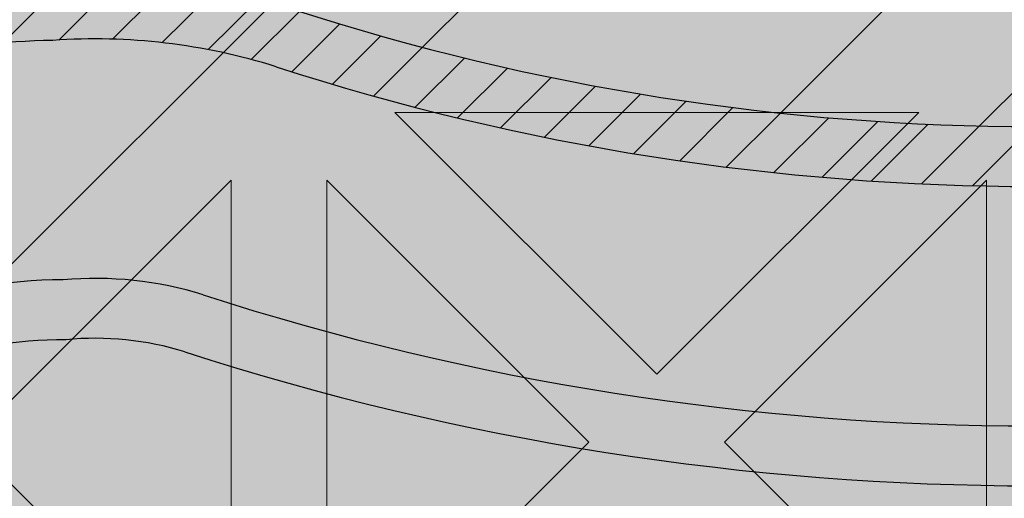
# Model space of a CAD drawing. Units: inches. Extents: x 844 to 2234, y 346 to 1084.
# Tile 54 of 93: x 1866.641 to 1869.26, y 692.527 to 693.802. Entities that reach past the tile are written whole.
import ezdxf

# ---------------------------------------------------------------- set-up
doc = ezdxf.new("R2010")
doc.units = ezdxf.units.IN
doc.header["$MEASUREMENT"] = 0
doc.layers.add('furniture', color=8, linetype='Continuous', lineweight=18)
doc.layers.add('RA-AP-01$0$INT', color=35, linetype='Continuous', lineweight=5)
doc.layers.add('RA-AP-01$0$FURN', color=3, linetype='Continuous')
doc.layers.add('RA-AP-01$0$WOOD', color=64, linetype='Continuous')

# ---------------------------------------------------------------- blocks, each defined once
blk = doc.blocks.new('A$C18D01794')
at = {"layer": 'RA-AP-01$0$INT'}
h = blk.add_hatch(color=256, dxfattribs=at)
h.paths.add_polyline_path([(4.585917135068449, -6.356712009588271), (4.555206456959269, -6.35671200958746), (4.555206456959137, -6.387422687716308), (4.874495778835233, -6.706712009592356), (4.90520645695423, -6.676001331474049)])
h.paths.add_polyline_path([(5.255206456948813, -6.387422687716306), (5.255206456948682, -6.356712009605972), (5.224495778822613, -6.356712009605161), (4.905206456953498, -6.676001331474273), (4.935917135072151, -6.706712009592924)])
h.paths.add_polyline_path([(4.935917135072559, -6.706712009592068), (4.905206456953564, -6.737422687710376), (5.255206456951813, -7.087422687708613), (5.255206456951549, -7.026001331471008)])
h.paths.add_polyline_path([(4.555206456956399, -7.026001331471013), (4.555206456956134, -7.087422687708616), (4.905206456953821, -6.737422687710943), (4.874495778835166, -6.70671200959229)])
h = blk.add_hatch(color=256, dxfattribs=at)
h.paths.add_polyline_path([(4.585917135068448, -6.356712009588273), (4.614201406330596, -6.356712009589021), (4.668846067270487, -6.411356670531338), (4.723490728212344, -6.356712009591912), (4.771774999457151, -6.35671200959319), (4.826419660396886, -6.411356670535356), (4.862780050090322, -6.374996280843536), (4.844495778842715, -6.356712009595112), (4.862780050090411, -6.356712009595595), (4.905206456960182, -6.399138416468211), (4.947632863832445, -6.356712009597838), (4.965917135079675, -6.356712009598322), (4.947632863831759, -6.374996280845421), (4.983993253523576, -6.411356670538857), (5.038637914464627, -6.356712009600247), (5.08692218571208, -6.356712009601523), (5.141566846649976, -6.411356670541852), (5.196211507589851, -6.356712009604411), (5.224495778822615, -6.356712009605161), (4.905206456953975, -6.676001331473793)])
h.paths.add_polyline_path([(4.895206456956031, -6.637717060225675), (4.895206456958921, -6.528427738347902), (4.840561796018589, -6.583072399285802)], flags=16)
h.paths.add_polyline_path([(4.915206456955638, -6.637717060226121), (4.969851117895509, -6.583072399288678), (4.915206456957609, -6.528427738348344)], flags=16)
h.paths.add_polyline_path([(4.826419660395175, -6.568930263661755), (4.881064321335613, -6.514285602723745), (4.771774999456703, -6.514285602720857)], flags=16)
h.paths.add_polyline_path([(4.983993253519558, -6.568930263665262), (5.038637914460456, -6.514285602726792), (4.929348592581548, -6.514285602724816)], flags=16)
h.paths.add_polyline_path([(4.881064321336025, -6.494285602723742), (4.826419660397532, -6.439640941782821), (4.771774999457062, -6.494285602720859)], flags=16)
h.paths.add_polyline_path([(4.929348592582019, -6.494285602724817), (5.038637914460982, -6.494285602726792), (4.983993253522945, -6.439640941786327)], flags=16)
h.paths.add_polyline_path([(4.895206456960191, -6.480143467100443), (4.895206456962115, -6.407422687715913), (4.876922185715016, -6.389138416467584), (4.840561796021581, -6.425498806159401)], flags=16)
h.paths.add_polyline_path([(4.915206456958487, -6.480143467100889), (4.969851117899527, -6.425498806162279), (4.933490728206909, -6.389138416468043), (4.9152064569598, -6.40742268771434)], flags=16)
h.paths.add_polyline_path([(4.757632863832376, -6.480143467096812), (4.812277524772842, -6.425498806158772), (4.757632863834348, -6.370854145217844)], flags=16)
h.paths.add_polyline_path([(4.737632863832376, -6.480143467096286), (4.737632863834348, -6.370854145217375), (4.682988202893906, -6.425498806155385)], flags=16)
h.paths.add_polyline_path([(5.05278005008503, -6.480143467103376), (5.052780050087917, -6.370854145224413), (4.998135389146995, -6.425498806162908)], flags=16)
h.paths.add_polyline_path([(5.072780050085024, -6.480143467103744), (5.127424711025931, -6.42549880616527), (5.072780050087916, -6.370854145224832)], flags=16)
h.paths.add_polyline_path([(4.935917135072783, -6.706712009592292), (5.255206456948811, -6.387422687716309), (5.255206456948932, -6.415706958964177), (5.200561796010279, -6.470351619902839), (5.255206456949403, -6.524996280841948), (5.25520645694961, -6.5732805520894), (5.200561796009787, -6.627925213029239), (5.236922185702417, -6.664285602721864), (5.255206456949919, -6.646001331474357), (5.255206456949998, -6.664285602721898), (5.212780050078687, -6.706712009592262), (5.25520645695036, -6.749138416463932), (5.255206456950438, -6.767422687711313), (5.236922185702424, -6.749138416463297), (5.200561796009796, -6.785498806155928), (5.255206456950753, -6.840143467096874), (5.25520645695096, -6.888427738341682), (5.200561796010322, -6.943072399282328), (5.255206456951428, -6.997717060223427), (5.255206456951547, -7.026001331471006)])
h.paths.add_polyline_path([(5.042988202883395, -6.785498806155427), (5.097632863823085, -6.840143467095101), (5.097632863822622, -6.730854145216193)], flags=16)
h.paths.add_polyline_path([(5.028846067259663, -6.771356670531693), (5.083490728198774, -6.716712009592573), (4.974201406321001, -6.716712009593042)], flags=16)
h.paths.add_polyline_path([(5.117632863823087, -6.840143467095186), (5.172277524762331, -6.785498806155926), (5.11763286382262, -6.730854145216225)], flags=16)
h.paths.add_polyline_path([(5.08349072819877, -6.696712009593886), (5.028846067259652, -6.642067348654775), (4.974201406320998, -6.696712009593438)], flags=16)
h.paths.add_polyline_path([(5.131774999446817, -6.854285602718917), (5.186419660386065, -6.799640941779662), (5.241064321325782, -6.854285602719365)], flags=17)
h.paths.add_polyline_path([(5.131774999446228, -6.716712009592374), (5.186419660386065, -6.771356670532194), (5.222780050079488, -6.734996280838764), (5.204495778832781, -6.716712009592063)], flags=16)
h.paths.add_polyline_path([(5.097632863822613, -6.682569873970264), (5.097632863823061, -6.573280552091354), (5.042988202883383, -6.627925213031044)], flags=16)
h.paths.add_polyline_path([(5.131774999446899, -6.874285602718915), (5.241064321325809, -6.874285602719364), (5.186419660386591, -6.928930263658598)], flags=17)
h.paths.add_polyline_path([(5.131774999446226, -6.696712009594078), (5.204495778830767, -6.696712009594374), (5.22278005007868, -6.67842773834687), (5.186419660386049, -6.642067348654249)], flags=16)
h.paths.add_polyline_path([(5.11763286382262, -6.682569873970225), (5.17227752476232, -6.627925213030515), (5.117632863823064, -6.573280552091267)], flags=16)
h.paths.add_polyline_path([(5.186419660386069, -6.613783077405491), (5.241064321325754, -6.559138416465795), (5.131774999446791, -6.559138416466263)], flags=16)
h.paths.add_polyline_path([(5.131774999446872, -6.539138416466263), (5.24106432132578, -6.539138416465794), (5.186419660386554, -6.484493755526573)], flags=16)
h.paths.add_polyline_path([(5.255206456951811, -7.08742268770861), (5.255206456951895, -7.106712009588038), (4.555206456956052, -7.106712009588038), (4.555206456956136, -7.087422687708617), (4.905206456953973, -6.737422687710788)])
h.paths.add_polyline_path([(4.983993253513404, -6.8444937555241), (4.92934859257295, -6.899138416462108), (5.03863791445186, -6.899138416465014)], flags=16)
h.paths.add_polyline_path([(4.969851117889988, -6.83035161990006), (4.915206456952556, -6.775706958960171), (4.915206456949648, -6.884996280837944)], flags=16)
h.paths.add_polyline_path([(4.929348592572535, -6.919138416462105), (4.983993253511019, -6.973783077403037), (5.038637914451496, -6.919138416465012)], flags=16)
h.paths.add_polyline_path([(5.052780050074912, -6.93328055208906), (4.998135389134438, -6.987925213027088), (5.052780050072919, -7.042569873968025)], flags=16)
h.paths.add_polyline_path([(5.07278005007491, -6.933280552089588), (5.072780050072918, -7.042569873968497), (5.127424711013374, -6.987925213030498)], flags=16)
h.paths.add_polyline_path([(4.89520645695295, -6.775706958959721), (4.840561796013067, -6.830351619897157), (4.895206456950961, -6.884996280837494)], flags=16)
h.paths.add_polyline_path([(4.915206456948365, -6.933280552085403), (4.915206456946434, -7.006001331471951), (4.933490728192729, -7.024285602719066), (4.969851117886972, -6.987925213026453)], flags=16)
h.paths.add_polyline_path([(4.881064321327021, -6.899138416461022), (4.82641966038902, -6.84449375552057), (4.771774999448108, -6.899138416459029)], flags=16)
h.paths.add_polyline_path([(4.895206456950073, -6.933280552084951), (4.840561796009022, -6.987925213023558), (4.876922185700835, -7.024285602716997), (4.895206456948749, -7.006001331469487)], flags=16)
h.paths.add_polyline_path([(4.983993253510392, -7.0020673486505), (4.947632863816944, -7.038427738342319), (4.965917135064043, -7.05671200959023), (5.038637914448995, -7.056712009591555)], flags=16)
h.paths.add_polyline_path([(4.881064321326543, -6.91913841646102), (4.771774999447578, -6.919138416459031), (4.826419660385607, -6.973783077399508)], flags=16)
h.paths.add_polyline_path([(4.905206456946447, -7.014285602717636), (4.862780050074785, -7.056712009588352), (4.947632863816685, -7.056712009589775)], flags=16)
h.paths.add_polyline_path([(5.14156684663679, -7.002067348654549), (5.086922185696452, -7.056712009592438), (5.196211507574223, -7.056712009594425)], flags=16)
h.paths.add_polyline_path([(4.8264196603837, -7.002067348646972), (4.771774999442643, -7.056712009585575), (4.8444957788276, -7.056712009587508), (4.862780050075511, -7.038427738340416)], flags=16)
h.paths.add_polyline_path([(4.812277524760289, -6.98792521302292), (4.757632863822258, -6.933280552082447), (4.757632863819352, -7.042569873961408)], flags=16)
h.paths.add_polyline_path([(4.73763286382226, -6.933280552082079), (4.682988202881349, -6.987925213020536), (4.737632863819352, -7.04256987396099)], flags=16)
h.paths.add_polyline_path([(4.723490728195188, -7.056712009584289), (4.668846067257299, -7.002067348643949), (4.614201406317417, -7.056712009581383)], flags=16)
h.paths.add_polyline_path([(4.597632863829262, -6.706712009592262), (4.555206456957951, -6.664285602721896), (4.555206456958029, -6.646001331474357), (4.573490728205535, -6.664285602721864), (4.609851117898167, -6.627925213029238), (4.555206456958338, -6.573280552089402), (4.555206456958546, -6.524996280841952), (4.60985111789767, -6.470351619902839), (4.555206456959015, -6.415706958964177), (4.555206456959138, -6.387422687716309), (4.874495778835167, -6.70671200959229), (4.5552064569564, -7.026001331471015), (4.555206456956523, -6.997717060223433), (4.609851117897629, -6.94307239928233), (4.555206456956988, -6.888427738341681), (4.555206456957198, -6.840143467096881), (4.609851117898153, -6.78549880615593), (4.573490728205528, -6.749138416463297), (4.555206456957507, -6.76742268771132), (4.555206456957585, -6.749138416463933)])
h.paths.add_polyline_path([(4.712780050085332, -6.730854145216195), (4.712780050084863, -6.840143467095105), (4.767424711024555, -6.785498806155427)], flags=16)
h.paths.add_polyline_path([(4.726922185709173, -6.716712009592573), (4.781566846648288, -6.771356670531693), (4.836211507586949, -6.716712009593043)], flags=16)
h.paths.add_polyline_path([(4.692780050085327, -6.730854145216225), (4.638135389145619, -6.785498806155928), (4.692780050084865, -6.840143467095185)], flags=16)
h.paths.add_polyline_path([(4.726922185709182, -6.696712009593886), (4.836211507586949, -6.696712009593436), (4.7815668466483, -6.642067348654773)], flags=16)
h.paths.add_polyline_path([(4.678637914461726, -6.71671200959237), (4.605917135075169, -6.716712009592063), (4.587632863828464, -6.734996280838766), (4.623993253521887, -6.771356670532195)], flags=16)
h.paths.add_polyline_path([(4.712780050085336, -6.68256987397026), (4.767424711024568, -6.627925213031042), (4.71278005008489, -6.573280552091352)], flags=16)
h.paths.add_polyline_path([(4.678637914461726, -6.696712009594076), (4.623993253521899, -6.642067348654247), (4.587632863829271, -6.67842773834687), (4.605917135077185, -6.696712009594376)], flags=16)
h.paths.add_polyline_path([(4.692780050085336, -6.682569873970228), (4.692780050084889, -6.573280552091267), (4.638135389145632, -6.627925213030515)], flags=16)
h.paths.add_polyline_path([(4.623993253521885, -6.799640941779662), (4.678637914461131, -6.854285602718915), (4.56934859258217, -6.854285602719365)], flags=17)
h.paths.add_polyline_path([(4.623993253521901, -6.613783077405509), (4.678637914461158, -6.559138416466263), (4.569348592582195, -6.559138416465795)], flags=16)
h.paths.add_polyline_path([(4.678637914461051, -6.874285602718915), (4.623993253521361, -6.928930263658598), (4.569348592582143, -6.874285602719364)], flags=17)
h.paths.add_polyline_path([(4.678637914461076, -6.539138416466263), (4.623993253521399, -6.484493755526573), (4.569348592582167, -6.539138416465796)], flags=16)
h = blk.add_hatch(color=256, dxfattribs=at)
h.paths.add_polyline_path([(4.969851117891331, -6.583072399286455), (4.915206456952669, -6.63771706022511), (4.915206456952222, -6.528427738347337)])
h.paths.add_polyline_path([(4.895206456953064, -6.637717060225108), (4.840561796014413, -6.583072399286448), (4.895206456953533, -6.528427738347335)])
h.paths.add_polyline_path([(4.826419660390684, -6.568930263662714), (4.771774999451003, -6.514285602723024), (4.881064321329913, -6.514285602723489)])
h.paths.add_polyline_path([(4.881064321329884, -6.494285602723492), (4.771774999450921, -6.494285602723024), (4.82641966039018, -6.439640941783778)])
h.paths.add_polyline_path([(4.895206456953734, -6.48014346709988), (4.840561796013912, -6.425498806160046), (4.876922185707337, -6.389138416466622), (4.895206456954043, -6.40742268771333)])
h.paths.add_polyline_path([(4.862780050082808, -6.374996280843689), (4.826419660390178, -6.411356670536314), (4.771774999450351, -6.356712009596481), (4.844495778835303, -6.356712009596181)])
h.paths.add_polyline_path([(4.812277524766446, -6.425498806160041), (4.757632863827191, -6.480143467099289), (4.757632863826741, -6.370854145220329)])
h.paths.add_polyline_path([(4.737632863827191, -6.480143467099214), (4.682988202887508, -6.425498806159518), (4.737632863826743, -6.370854145220299)])
h.paths.add_polyline_path([(4.668846067263777, -6.41135667053579), (4.614201406325123, -6.356712009597128), (4.723490728202894, -6.356712009596675)])
h.paths.add_polyline_path([(4.905206456953846, -6.399138416467422), (4.862780050082654, -6.356712009596229), (4.947632863824561, -6.356712009595756)])
h.paths.add_polyline_path([(4.915206456952028, -6.480143467099882), (4.91520645695173, -6.407422687715346), (4.933490728199234, -6.389138416467428), (4.96985111789186, -6.425498806160055)])
h.paths.add_polyline_path([(5.038637914454841, -6.494285602723048), (4.929348592575874, -6.494285602723497), (4.983993253515593, -6.439640941783787)])
h.paths.add_polyline_path([(4.983993253515065, -6.568930263662725), (4.929348592575849, -6.514285602723495), (5.038637914454755, -6.514285602723045)])
h.paths.add_polyline_path([(5.052780050079843, -6.480143467099317), (4.998135389140595, -6.425498806160058), (5.052780050080309, -6.370854145220356)])
h.paths.add_polyline_path([(4.983993253516868, -6.411356670536324), (4.947632863824241, -6.374996280843694), (4.965917135071747, -6.356712009596188), (5.038637914456701, -6.356712009596504)])
h.paths.add_polyline_path([(5.127424711019533, -6.425498806159557), (5.072780050079843, -6.480143467099239), (5.07278005008031, -6.370854145220326)])
h.paths.add_polyline_path([(5.141566846643269, -6.411356670535829), (5.086922185704154, -6.356712009596707), (5.196211507581929, -6.356712009597176)])
for p, q in [((4.905206456953975, -6.676001331473793), (4.585917135071132, -6.356712009590955)), ((4.737632863834348, -6.370854145217375), (4.682988202893906, -6.425498806155385)), ((4.737632863832376, -6.480143467096285), (4.737632863834348, -6.370854145217375)), ((4.757632863832376, -6.48014346709681), (4.757632863834348, -6.370854145217847)), ((4.757632863834348, -6.370854145217847), (4.812277524772842, -6.425498806158774)), ((4.840561796021581, -6.425498806159403), (4.876922185715016, -6.389138416467584)), ((4.895206456962113, -6.407422687715495), (4.895206456960191, -6.480143467100447)), ((4.682988202893908, -6.425498806155387), (4.737632863832376, -6.480143467096285)), ((4.757632863832376, -6.48014346709681), (4.812277524772842, -6.425498806158774)), ((4.895206456960191, -6.480143467100447), (4.840561796021581, -6.425498806159401)), ((4.771774999457064, -6.494285602720857), (4.826419660397532, -6.439640941782821)), ((4.881064321336027, -6.494285602723744), (4.826419660397532, -6.439640941782821)), ((4.771774999457064, -6.494285602720857), (4.881064321336027, -6.494285602723744))]:
    blk.add_line(p, q, dxfattribs=at)
blk = doc.blocks.new('A$C32926AE1')
at = {"layer": 'RA-AP-01$0$WOOD'}
h = blk.add_hatch(color=256, dxfattribs=at)
h.dxf.hatch_style = 1
h.paths.add_polyline_path([(5.157430609644524, 4.573483066760929, -0.1009492694046607), (5.155401577623758, 4.593365984175333, -0.1842662638101597), (5.172249623284174, 4.638795604568598, 0.2056608120311276), (5.179560981299304, 4.661316324430096, 0.3614336704623542), (5.134352340494423, 4.706524965234944, 0.2056608120311297), (5.111831620632933, 4.699213607219793, -0.1842662638101113), (5.066402000239693, 4.682365561559342, -0.1055311479399994), (5.045656153913092, 4.68467289944697, 0.1567636581983829), (4.763886414745334, 4.684672899446966, -0.1055311479399895), (4.743140568418733, 4.68236556155934, -0.1842662638100833), (4.6977109480255, 4.69921360721979, 0.2056608120302612), (4.675190228164109, 4.706524965234949, 0.3614336704708441), (4.629981587358889, 4.66131632442871, 0.2056608120245944), (4.637292945374126, 4.638795604567974, -0.1842662638101024), (4.654140991034615, 4.59336598417475, -0.1009492694055169), (4.652111959013835, 4.573483066760181, 0.021410119221476), (4.629748025606143, 4.156712009541676, 0.0214101192214795), (4.652111959013809, 3.739940952323101, -0.1009492694059586), (4.654140991034615, 3.720058034908448, -0.1842662638100975), (4.637292945374126, 3.674628414515226, 0.2056608120245705), (4.629981587358889, 3.652107694654492, 0.3614336704708879), (4.675190228164113, 3.606899053848249, 0.2056608120302384), (4.697710948025501, 3.614210411863408, -0.1842662638100995), (4.743140568418738, 3.63105845752386, -0.1055311479402541), (4.763886414745388, 3.628751119636215, 0.1567636581983776), (5.045656153913137, 3.628751119636244, -0.1055311479397538), (5.066402000239692, 3.631058457523857, -0.1842662638101067), (5.111831620632931, 3.614210411863407, 0.2056608120310924), (5.134352340494417, 3.606899053848256, 0.3614336704624001), (5.179560981299307, 3.652107694653103, 0.2056608120311314), (5.172249623284175, 3.6746284145146, -0.1842662638101402), (5.155401577623758, 3.72005803490786, -0.1009492694051366), (5.15743060964455, 3.739940952322354, 0.0214101192215073), (5.179794543052287, 4.156712009541468, 0.0214101192215252)])
h.paths.add_polyline_path([(4.639748609479751, 4.156712009541513, 0.0213537860821624), (4.661970494867118, 3.741887061152232, -0.094075836301374), (4.664143710413708, 3.7196126951003, -0.1824818158568985), (4.644813765429836, 3.668037719127816, 0.2056608120245319), (4.639939526753007, 3.653023905887301, 0.3614336704710246), (4.676106439397173, 3.616856993242342, 0.2056608120302234), (4.691120252638095, 3.621731231919122, -0.1824818158602558), (4.742695228611606, 3.641061176902986, -0.1029891339458722), (4.766991894714349, 3.638256818950944, 0.156709409989566), (5.042550673941472, 3.638256818950105, -0.102989133958497), (5.066847340047078, 3.641061176902949, -0.1824818158594995), (5.118422316020358, 3.621731231919103, 0.2056608120311416), (5.133436129261316, 3.616856993242346, 0.3614336704621468), (5.169603041905217, 3.653023905886178, 0.2056608120310986), (5.164728803228477, 3.668037719127177, -0.1824818158565612), (5.145398858244737, 3.719612695099578, -0.0940758363009313), (5.147572073791232, 3.741887061151398, 0.0213537860822023), (5.169793959178681, 4.156712009541451, 0.0213537860822226), (5.147572073791203, 4.571536957931898, -0.0940758363005034), (5.145398858244737, 4.59381132398362, -0.1824818158565587), (5.164728803228476, 4.645386299956021, 0.2056608120311045), (5.169603041905216, 4.66040011319702, 0.3614336704621845), (5.133436129261313, 4.696567025840856, 0.2056608120310773), (5.118422316020359, 4.691692787164098, -0.182481815859508), (5.066847340047078, 4.67236284218025, -0.1029891339584606), (5.04255067394148, 4.675167200133092, 0.156709409989566), (4.766991894714357, 4.675167200132257, -0.1029891339458842), (4.742695228611611, 4.672362842180213, -0.1824818158602725), (4.691120252638095, 4.691692787164077, 0.2056608120302152), (4.676106439397174, 4.696567025840858, 0.3614336704710363), (4.639939526753005, 4.660400113195899, 0.2056608120245495), (4.644813765429837, 4.645386299955384, -0.1824818158568934), (4.664143710413708, 4.593811323982902, -0.0940758363009187), (4.661970494867149, 4.571536957931074, 0.021353786082177)], flags=16)
h.paths.add_polyline_path([(5.129794543052235, 4.432167055276933, -0.0141661062790638), (5.130152669293814, 4.156927903047693, -0.0141661062790647), (5.129794543052234, 3.881688750818433, -0.0785247771143638), (5.10979738006795, 3.755143611847103, 0.0945969212073497), (5.105408519571111, 3.717898134952927, 0.1043170707844957), (5.116074640131521, 3.670385395016088, 0.1043170707864965), (5.068561900193738, 3.681051515576561, 0.09459692119553), (5.031316423304057, 3.676662655080835, -0.1580239521427272), (4.778226145355827, 3.676662655080367, 0.0945969211986668), (4.740980668464973, 3.681051515576592, 0.1043170707882822), (4.693467928526415, 3.670385395015844, 0.1043170707867916), (4.704134049087309, 3.717898134953662, 0.0945969211972894), (4.69974518859162, 3.755143611844042, -0.0785247771163196), (4.679748025606343, 3.881688750818406, -0.0141661062790663), (4.679389899364763, 4.156927903047693, -0.0141661062790672), (4.679748025606343, 4.432167055276998, -0.0785247771163064), (4.699745188591625, 4.55871219425134, 0.094596921197333), (4.704134049087308, 4.595957671141738, 0.1043170707867205), (4.693467928526416, 4.643470411079523, 0.1043170707882628), (4.740980668464965, 4.632804290518776, 0.0945969211988114), (4.778226145355874, 4.637193151015016, -0.158023952142669), (5.031316423304015, 4.637193151014546, 0.0945969211956361), (5.068561900193736, 4.632804290518806, 0.1043170707864979), (5.11607464013152, 4.643470411079278, 0.1043170707844617), (5.105408519571112, 4.595957671142455, 0.0945969212074597), (5.109797380067959, 4.558712194248236, -0.0785247771143467)], flags=0)
h.paths.add_polyline_path([(5.119794532311105, 4.432259799204851, -0.0142000800617244), (5.120156169157484, 4.156927903047701, -0.0142000800617277), (5.119794532311105, 3.881596006890482, -0.0784894509520253), (5.100273383573699, 3.758192358677797, 0.0940138827242913), (5.095413455884425, 3.717477693979438, 0.0606271852308753), (5.099615656341024, 3.686844378806616, 0.0606271852322524), (5.068982341167493, 3.691046579263239, 0.0940138827010453), (5.028267676478798, 3.686186651576848, -0.1580706864508061), (4.781274892180912, 3.686186651576435, 0.0940138827026903), (4.740560227491556, 3.691046579263279, 0.0606271852339895), (4.709926912317155, 3.686844378806508, 0.0606271852329405), (4.714129112773991, 3.717477693980356, 0.094013882701304), (4.709269185087677, 3.758192358669163, -0.0784894509577193), (4.689748036347473, 3.881596006890469, -0.014200080061729), (4.689386399501094, 4.156927903047709, -0.0142000800617217), (4.689748036347473, 4.432259799204808, -0.078489450957724), (4.709269185087651, 4.555663447426125, 0.0940138827014585), (4.714129112773992, 4.596378112114996, 0.0606271852329731), (4.709926912317154, 4.62701142728886, 0.0606271852340196), (4.74056022749157, 4.622809226832087, 0.0940138827024997), (4.781274892180847, 4.627669154518912, -0.1580706864508359), (5.028267676478777, 4.627669154518526, 0.0940138827010946), (5.068982341167492, 4.622809226832129, 0.060627185232254), (5.099615656341024, 4.627011427288751, 0.0606271852308727), (5.095413455884425, 4.59637811211593, 0.0940138827241088), (5.100273383573675, 4.555663447417647, -0.0784894509520978)], flags=0)
h.paths.add_polyline_path([(5.06978912287499, 4.430218106756144, -0.014241683694547), (5.070173729147532, 4.156927903047672, -0.0142416836945458), (5.06978912287499, 3.883637699339223, -0.0800609523125196), (5.052662118612511, 3.773463122773442, 0.0526421978001116), (5.04590916754064, 3.740550867606997, 0.0526421977992423), (5.012996912374707, 3.73379791653534, -0.1583028414718258), (4.796545656286308, 3.73379791653451, 0.0526421978034211), (4.763633401117837, 3.740550867607021, 0.0526421978018622), (4.756880450045755, 3.773463122774558, -0.0800609523117106), (4.739753445783639, 3.883637699339268, -0.0142416836945435), (4.739368839511098, 4.156927903047671, -0.0142416836945477), (4.739753445783639, 4.430218106756155, -0.0800609523116345), (4.75688045004574, 4.540392683320762, 0.052642197801941), (4.763633401117837, 4.573304938488346, 0.0526421978035071), (4.796545656286361, 4.580057889560873, -0.1583028414717561), (5.012996912374669, 4.580057889560039, 0.0526421977993048), (5.04590916754064, 4.57330493848837, 0.0526421978002057), (5.052662118612529, 4.540392683321868, -0.080060952312477)], flags=0)
h.paths.add_polyline_path([(5.049789715110557, 4.43038092723357, -0.0143097550741839), (5.05018085590259, 4.156927903047715, -0.0143097550741854), (5.049789715110558, 3.883474878861827, -0.0800685599149176), (5.03362098255317, 3.779581877367999, 0.0306258898956367), (5.028241146483733, 3.758218888663947, 0.0306258898977031), (5.006878157778253, 3.75283905259408, -0.1583983521624096), (4.802664410878162, 3.752839052594731, 0.0306258898946014), (4.781301422174808, 3.758218888663924, 0.0306258898967912), (4.775921586105202, 3.779581877368794, -0.080068559914251), (4.759752853548071, 3.883474878861786, -0.0143097550741854), (4.759361712756037, 4.156927903047671, -0.0143097550741854), (4.759752853548071, 4.430380927233557, -0.0800685599142479), (4.775921586105193, 4.534273928726546, 0.0306258898968306), (4.781301422174808, 4.555636917431444, 0.0306258898945754), (4.802664410878143, 4.561016753500631, -0.1583983521624168), (5.006878157778244, 4.561016753501291, 0.0306258898977177), (5.028241146483733, 4.555636917431421, 0.0306258898958182), (5.03362098255321, 4.534273928727244, -0.080068559914796)], flags=0)
h.paths.add_polyline_path([(4.999766070382627, 4.428171244713864, -0.0143443147609634), (5.000198441819402, 4.156927903047689, -0.0143443147609612), (4.999766070382627, 3.885684561381556, -0.0784641635803329), (4.987356730658798, 3.799103304488872, -0.1506053783831347), (4.822185837999821, 3.79910330448882, -0.0784641635803318), (4.809776498276007, 3.885684561381509, -0.014344314760963), (4.809344126839227, 4.156927903047677, -0.0143443147609645), (4.809776498276007, 4.428171244713873, -0.0784641635803192), (4.822185837999822, 4.514752501606549, -0.1506053783831338), (4.987356730658798, 4.514752501606494, -0.078464163580285)], flags=0)
h.paths.add_polyline_path([(4.979755254238824, 4.42764379880488, -0.0143772539198268), (4.980205517789977, 4.156927903047693, -0.0143772539198275), (4.979755254238824, 3.886212007290489, -0.0689242507424422), (4.971183264704897, 3.815276770442801, -0.1296645318904179), (4.838359303953726, 3.815276770442746, -0.0689242507424186), (4.829787314419809, 3.886212007290419, -0.0143772539198292), (4.829337050868653, 4.156927903047653, -0.0143772539198325), (4.829787314419809, 4.427643798804946, -0.0689242507424211), (4.838359303953725, 4.498579035652621, -0.1296645318904187), (4.971183264704897, 4.498579035652565, -0.0689242507424401)], flags=0)
h = blk.add_hatch(color=256, dxfattribs=at)
h.dxf.hatch_style = 1
h.paths.add_polyline_path([(5.145398858244737, 4.59381132398362, -0.1824818158565616), (5.164728803228476, 4.645386299956021, 0.2056608120311045), (5.169603041905216, 4.66040011319702, 0.3614336704621845), (5.133436129261313, 4.696567025840856, 0.2056608120310773), (5.118422316020359, 4.691692787164098, -0.182481815859508), (5.066847340047078, 4.67236284218025, -0.1029891339584606), (5.04255067394148, 4.675167200133092, 0.156709409989566), (4.766991894714357, 4.675167200132257, -0.1029891339458842), (4.742695228611611, 4.672362842180213, -0.1824818158602725), (4.691120252638095, 4.691692787164077, 0.2056608120302152), (4.676106439397174, 4.696567025840858, 0.3614336704710363), (4.639939526753005, 4.660400113195899, 0.2056608120245495), (4.644813765429837, 4.645386299955384, -0.1824818158568934), (4.664143710413708, 4.593811323982902, -0.0940758363009187), (4.661970494867149, 4.571536957931074, 0.0213537860821772), (4.639748609479751, 4.156712009541507, 0.0213537860821625), (4.661970494867119, 3.741887061152226, -0.0940758363013071), (4.664143710413708, 3.719612695100309, -0.1824818158569294), (4.644813765429836, 3.668037719127816, 0.2056608120245319), (4.639939526753007, 3.653023905887301, 0.3614336704710246), (4.676106439397173, 3.616856993242342, 0.2056608120302234), (4.691120252638095, 3.621731231919122, -0.1824818158602558), (4.742695228611606, 3.641061176902986, -0.1029891339458722), (4.766991894714349, 3.638256818950944, 0.156709409989566), (5.042550673941472, 3.638256818950105, -0.102989133958497), (5.066847340047078, 3.641061176902949, -0.1824818158594995), (5.118422316020358, 3.621731231919103, 0.2056608120311416), (5.133436129261316, 3.616856993242346, 0.3614336704621468), (5.169603041905217, 3.653023905886178, 0.2056608120310986), (5.164728803228477, 3.668037719127177, -0.1824818158565612), (5.145398858244737, 3.719612695099578, -0.0940758363009313), (5.147572073791232, 3.741887061151398, 0.0213537860822023), (5.169793959178681, 4.156712009541451, 0.0213537860822226), (5.147572073791203, 4.571536957931898, -0.0940758363004996)])
h.paths.add_polyline_path([(5.109797380067958, 4.55871219424824, -0.0785247771143472), (5.129794543052234, 4.432167055276936, -0.0141661062790644), (5.130152669293814, 4.156927903047685, -0.014166106279066), (5.129794543052234, 3.881688750818401, -0.0785247771143517), (5.109797380067946, 3.755143611847092, 0.0945969212073132), (5.105408519571111, 3.717898134952929, 0.1043170707844995), (5.116074640131521, 3.670385395016088, 0.1043170707864965), (5.068561900193738, 3.681051515576561, 0.09459692119553), (5.031316423304057, 3.676662655080835, -0.1580239521427272), (4.778226145355827, 3.676662655080367, 0.0945969211986668), (4.740980668464973, 3.681051515576592, 0.1043170707882822), (4.693467928526415, 3.670385395015844, 0.1043170707867916), (4.704134049087309, 3.717898134953662, 0.0945969211972894), (4.69974518859162, 3.755143611844042, -0.0785247771163196), (4.679748025606343, 3.881688750818406, -0.0141661062790663), (4.679389899364763, 4.156927903047693, -0.0141661062790672), (4.679748025606343, 4.432167055276998, -0.0785247771163064), (4.699745188591625, 4.55871219425134, 0.094596921197333), (4.704134049087308, 4.595957671141738, 0.1043170707867205), (4.693467928526416, 4.643470411079523, 0.1043170707882628), (4.740980668464965, 4.632804290518776, 0.0945969211988114), (4.778226145355874, 4.637193151015016, -0.158023952142669), (5.031316423304015, 4.637193151014546, 0.0945969211956361), (5.068561900193736, 4.632804290518806, 0.1043170707864979), (5.11607464013152, 4.643470411079278, 0.1043170707844617), (5.105408519571112, 4.595957671142455, 0.0945969212074504)], flags=16)
h.paths.add_polyline_path([(5.100273383573655, 4.55566344741771, -0.0784894509521388), (5.119794532311105, 4.432259799204852, -0.0142000800617252), (5.120156169157484, 4.156927903047686, -0.014200080061726), (5.119794532311105, 3.881596006890502, -0.0784894509520446), (5.100273383573696, 3.758192358677786, 0.0940138827242721), (5.095413455884425, 3.717477693979436, 0.0606271852308692), (5.099615656341024, 3.686844378806616, 0.0606271852322522), (5.068982341167493, 3.691046579263239, 0.0940138827010453), (5.028267676478798, 3.686186651576848, -0.1580706864508061), (4.781274892180912, 3.686186651576435, 0.0940138827026903), (4.740560227491556, 3.691046579263279, 0.0606271852339895), (4.709926912317155, 3.686844378806508, 0.0606271852329405), (4.714129112773991, 3.717477693980356, 0.094013882701304), (4.709269185087677, 3.758192358669163, -0.0784894509577193), (4.689748036347473, 3.881596006890469, -0.014200080061729), (4.689386399501094, 4.156927903047709, -0.0142000800617217), (4.689748036347473, 4.432259799204808, -0.078489450957724), (4.709269185087651, 4.555663447426125, 0.0940138827014585), (4.714129112773992, 4.596378112114996, 0.0606271852329731), (4.709926912317154, 4.62701142728886, 0.0606271852340196), (4.74056022749157, 4.622809226832087, 0.0940138827024997), (4.781274892180847, 4.627669154518912, -0.1580706864508359), (5.028267676478777, 4.627669154518526, 0.0940138827010946), (5.068982341167492, 4.622809226832129, 0.060627185232254), (5.099615656341024, 4.627011427288751, 0.0606271852308727), (5.095413455884425, 4.59637811211593, 0.094013882723957)], flags=0)
h.paths.add_polyline_path([(5.04590916754064, 4.57330493848837, 0.0526421978002057), (5.052662118612529, 4.540392683321868, -0.0800609523124783), (5.06978912287499, 4.430218106756142, -0.0142416836945469), (5.070173729147532, 4.156927903047672, -0.0142416836945458), (5.06978912287499, 3.883637699339223, -0.0800609523125196), (5.052662118612511, 3.773463122773442, 0.0526421978001116), (5.04590916754064, 3.740550867606997, 0.0526421977992423), (5.012996912374707, 3.73379791653534, -0.1583028414718258), (4.796545656286308, 3.73379791653451, 0.0526421978034211), (4.763633401117837, 3.740550867607021, 0.0526421978018622), (4.756880450045755, 3.773463122774558, -0.0800609523117106), (4.739753445783639, 3.883637699339268, -0.0142416836945435), (4.739368839511098, 4.156927903047671, -0.0142416836945477), (4.739753445783639, 4.430218106756155, -0.0800609523116345), (4.75688045004574, 4.540392683320762, 0.052642197801941), (4.763633401117837, 4.573304938488346, 0.0526421978035071), (4.796545656286361, 4.580057889560873, -0.1583028414717561), (5.012996912374669, 4.580057889560039, 0.0526421977993048)], flags=0)
h.paths.add_polyline_path([(5.028241146483733, 4.555636917431422, 0.0306258898956949), (5.033620982553182, 4.534273928727329, -0.0800685599148649), (5.049789715110557, 4.430380927233569, -0.0143097550741839), (5.05018085590259, 4.156927903047715, -0.0143097550741854), (5.049789715110558, 3.883474878861827, -0.0800685599149176), (5.03362098255317, 3.779581877367999, 0.0306258898956367), (5.028241146483733, 3.758218888663947, 0.0306258898977031), (5.006878157778253, 3.75283905259408, -0.1583983521624096), (4.802664410878162, 3.752839052594731, 0.0306258898946014), (4.781301422174808, 3.758218888663924, 0.0306258898967912), (4.775921586105202, 3.779581877368794, -0.080068559914251), (4.759752853548071, 3.883474878861786, -0.0143097550741854), (4.759361712756037, 4.156927903047671, -0.0143097550741854), (4.759752853548071, 4.430380927233557, -0.0800685599142479), (4.775921586105193, 4.534273928726546, 0.0306258898968306), (4.781301422174808, 4.555636917431444, 0.0306258898945754), (4.802664410878143, 4.561016753500631, -0.1583983521624168), (5.006878157778244, 4.561016753501291, 0.0306258898977174)], flags=0)
h.paths.add_polyline_path([(4.987356730658798, 4.514752501606494, -0.0784641635803018), (4.999766070382627, 4.428171244713845, -0.0143443147609637), (5.000198441819402, 4.156927903047665, -0.0143443147609622), (4.999766070382628, 3.885684561381514, -0.0784641635802952), (4.987356730658797, 3.799103304488872, -0.1506053783831338), (4.822185837999821, 3.799103304488819, -0.0784641635803342), (4.809776498276007, 3.885684561381512, -0.0143443147609628), (4.809344126839227, 4.156927903047676, -0.0143443147609646), (4.809776498276007, 4.428171244713873, -0.0784641635803192), (4.822185837999822, 4.514752501606549, -0.1506053783831338)], flags=0)
h.paths.add_polyline_path([(4.971183264704897, 4.498579035652566, -0.0689242507424384), (4.979755254238824, 4.427643798804883, -0.0143772539198276), (4.980205517789977, 4.15692790304768, -0.0143772539198258), (4.979755254238823, 3.88621200729051, -0.0689242507424628), (4.971183264704897, 3.815276770442801, -0.129664531890417), (4.838359303953726, 3.815276770442746, -0.0689242507424186), (4.829787314419809, 3.886212007290419, -0.0143772539198292), (4.829337050868653, 4.156927903047653, -0.0143772539198325), (4.829787314419809, 4.427643798804946, -0.0689242507424211), (4.838359303953725, 4.498579035652621, -0.1296645318904187)], flags=0)
h = blk.add_hatch(dxfattribs=at)
h.set_pattern_fill('ANSI31', color=256, scale=0.05, style=0)
h.set_pattern_definition([(45, (0, 0), (-0.0044194173824159, 0.0044194173824159), [])])
h.paths.add_polyline_path([(5.130152669293814, 4.156927903047704, 0.0141661062790657), (5.129794543052234, 4.432167055276982, 0.0777827904001433), (5.110168979996553, 4.557559993161921, -0.0976515123401879), (5.105408519571111, 4.595957671142454, -0.1043170707844687), (5.116074640131522, 4.64347041107928), (5.099615656341024, 4.627011427288751, 0.0606271852308727), (5.095413455884425, 4.59637811211593, 0.0940138827241088), (5.100273383573675, 4.555663447417647, -0.0784894509520972), (5.119794532311105, 4.432259799204852, -0.0142000800617252), (5.120156169157484, 4.156927903047686, -0.014200080061726), (5.119794532311105, 3.881596006890502, -0.0784894509520446), (5.100273383573696, 3.758192358677786, 0.0940138827242721), (5.095413455884425, 3.717477693979436, 0.0606271852308692), (5.099615656341024, 3.686844378806616), (5.116074640131519, 3.67038539501609, -0.1043170707844594), (5.105408519571112, 3.717898134952912, -0.0976515123401594), (5.11016897999655, 3.756295812933435, 0.0777827904001654), (5.129794543052234, 3.881688750818409, 0.0141661062790665)])
h.paths.add_polyline_path([(5.030164222210597, 3.676291055149937, -0.0976515123472002), (5.068561900193739, 3.681051515576561, -0.1043170707864927), (5.116074640131521, 3.670385395016088), (5.099615656341024, 3.686844378806616, 0.0606271852322522), (5.068982341167493, 3.691046579263239, 0.0940138827010453), (5.028267676478798, 3.686186651576848, -0.1580706864508061), (4.781274892180912, 3.686186651576435, 0.0940138827026903), (4.740560227491556, 3.691046579263279, 0.0606271852339913), (4.709926912317154, 3.686844378806508), (4.693467928526416, 3.670385395015845, -0.1043170707882796), (4.740980668464973, 3.681051515576592, -0.0976515123427246), (4.779378346446416, 3.676291055150394, 0.156512506893803)])
h.paths.add_polyline_path([(4.689748036347473, 3.881596006890472, -0.014200080061729), (4.689386399501094, 4.156927903047712, -0.0142000800617195), (4.689748036347473, 4.432259799204768, -0.078489450957742), (4.709269185087648, 4.555663447426114, 0.0940138827014821), (4.714129112773992, 4.596378112114995, 0.0606271852329748), (4.709926912317154, 4.62701142728886), (4.693467928526414, 4.643470411079524, -0.1043170707867939), (4.704134049087309, 4.595957671141706, -0.09765151234893), (4.699373588660725, 4.557559993157876, 0.0777827903975372), (4.679748025606343, 4.432167055276987, 0.0141661062790675), (4.679389899364763, 4.156927903047675, 0.0141661062790641), (4.679748025606343, 3.88168875081843, 0.0777827903975637), (4.699373588660724, 3.756295812937497, -0.0976515123490278), (4.704134049087308, 3.717898134953629, -0.1043170707867196), (4.693467928526416, 3.670385395015845), (4.709926912317155, 3.686844378806508, 0.0606271852329413), (4.714129112773991, 3.717477693980357, 0.0940138827013084), (4.709269185087676, 3.758192358669166, -0.0784894509577192)])
h.paths.add_polyline_path([(4.779378346446434, 4.63756475094498, -0.0976515123427943), (4.740980668464964, 4.632804290518776, -0.1043170707882609), (4.693467928526416, 4.643470411079523), (4.709926912317154, 4.62701142728886, 0.0606271852340196), (4.74056022749157, 4.622809226832087, 0.0940138827024997), (4.781274892180847, 4.627669154518912, -0.1580706864508359), (5.028267676478777, 4.627669154518526, 0.0940138827010946), (5.068982341167492, 4.622809226832129, 0.060627185232254), (5.099615656341024, 4.627011427288751), (5.116074640131521, 4.643470411079279, -0.1043170707865022), (5.068561900193735, 4.632804290518806, -0.0976515123475899), (5.030164222210446, 4.637564750945479, 0.1565125068936924)])
h = blk.add_hatch(dxfattribs=at)
h.set_pattern_fill('ANSI32', color=256, scale=0.2, style=0)
h.set_pattern_definition([(45, (0, 0), (-0.0530330085889911, 0.0530330085889911), []), (45, (0.035355339, 0), (-0.0530330085889911, 0.0530330085889911), [])])
h.paths.add_polyline_path([(5.119794532311105, 4.432259799204823, 0.0777015974868765), (5.10065834347252, 4.554469821747928, -0.0968902511992216), (5.095413455884425, 4.596378112115931, -0.060627185230871), (5.099615656341024, 4.627011427288751, -0.060627185232254), (5.068982341167492, 4.622809226832129, -0.0968902512198245), (5.027074050790956, 4.628054114423209, 0.1564657949319105), (4.782468517866163, 4.628054114422785, -0.0968902512152247), (4.740560227491555, 4.622809226832088, -0.0606271852339878), (4.709926912317155, 4.627011427288859, -0.0606271852329413), (4.714129112773991, 4.596378112115011, -0.0968902512205338), (4.708884225182929, 4.554469821738175, 0.0777015974804443), (4.689748036347473, 4.43225979920482, 0.0142000800617215), (4.689386399501094, 4.156927903047726, 0.0142000800617273), (4.689748036347473, 3.88159600689052, 0.077701597480541), (4.708884225182985, 3.759385984357019, -0.096890251220082), (4.714129112773992, 3.717477693980371, -0.0606271852329731), (4.709926912317154, 3.686844378806507, -0.060627185233988), (4.740560227491554, 3.691046579263279, -0.0968902512152569), (4.782468517866175, 3.685801691672578, 0.1564657949319236), (5.027074050790988, 3.685801691672169, -0.0968902512197451), (5.068982341167491, 3.691046579263239, -0.0606271852322557), (5.099615656341024, 3.686844378806616, -0.0606271852308727), (5.095413455884425, 3.717477693979438, -0.0968902511991229), (5.100658343472507, 3.7593859843474, 0.0777015974868745), (5.119794532311105, 3.8815960068905, 0.014200080061726), (5.120156169157484, 4.156927903047685, 0.0142000800617238)])
h.paths.add_polyline_path([(5.070173729147531, 4.156927903047684, -0.0142416836945481), (5.06978912287499, 3.883637699339191, -0.0800609523125107), (5.052662118612505, 3.773463122773424, 0.0526421978000811), (5.04590916754064, 3.740550867606997, 0.0526421977993214), (5.012996912374658, 3.733797916535325, -0.1583028414717916), (4.796545656286304, 3.733797916534512, 0.0526421978034138), (4.763633401117837, 3.740550867607021, 0.0526421978018622), (4.756880450045755, 3.773463122774558, -0.0800609523117106), (4.739753445783639, 3.883637699339268, -0.0142416836945435), (4.739368839511098, 4.156927903047671, -0.0142416836945477), (4.739753445783639, 4.430218106756155, -0.0800609523116345), (4.75688045004574, 4.540392683320762, 0.052642197801941), (4.763633401117837, 4.573304938488346, 0.0526421978035071), (4.796545656286361, 4.580057889560873, -0.1583028414717561), (5.012996912374669, 4.580057889560039, 0.0526421977993048), (5.04590916754064, 4.57330493848837, 0.0526421978002057), (5.052662118612529, 4.540392683321868, -0.0800609523124783), (5.06978912287499, 4.430218106756142, -0.0142416836945463)], flags=16)
h.paths.add_polyline_path([(5.050180855902591, 4.156927903047686, -0.0143097550741856), (5.049789715110558, 3.883474878861795, -0.0800685599148126), (5.033620982553202, 3.7795818773681, 0.0306258898957837), (5.028241146483733, 3.758218888663947, 0.0306258898977031), (5.006878157778253, 3.75283905259408, -0.1583983521624096), (4.802664410878162, 3.752839052594731, 0.0306258898946014), (4.781301422174808, 3.758218888663924, 0.0306258898967912), (4.775921586105202, 3.779581877368794, -0.080068559914251), (4.759752853548071, 3.883474878861786, -0.0143097550741854), (4.759361712756037, 4.156927903047671, -0.0143097550741854), (4.759752853548071, 4.430380927233557, -0.0800685599142479), (4.775921586105193, 4.534273928726546, 0.0306258898968306), (4.781301422174808, 4.555636917431444, 0.0306258898945754), (4.802664410878143, 4.561016753500631, -0.1583983521624168), (5.006878157778244, 4.561016753501291, 0.0306258898977177), (5.028241146483733, 4.555636917431421, 0.0306258898958182), (5.03362098255321, 4.534273928727244, -0.0800685599147973), (5.049789715110557, 4.430380927233568, -0.0143097550741854)], flags=0)
h.paths.add_polyline_path([(5.000198441819402, 4.15692790304769, -0.0143443147609622), (4.999766070382627, 3.885684561381539, -0.0784641635803169), (4.987356730658798, 3.799103304488873, -0.1506053783831347), (4.822185837999821, 3.79910330448882, -0.0784641635803318), (4.809776498276007, 3.885684561381509, -0.014344314760963), (4.809344126839227, 4.156927903047677, -0.0143443147609645), (4.809776498276007, 4.428171244713873, -0.0784641635803192), (4.822185837999822, 4.514752501606549, -0.1506053783831338), (4.987356730658798, 4.514752501606494, -0.0784641635803018), (4.999766070382627, 4.428171244713845, -0.0143443147609624)], flags=0)
h.paths.add_polyline_path([(4.980205517789976, 4.156927903047707, -0.0143772539198295), (4.979755254238824, 3.886212007290466, -0.06892425074242), (4.971183264704897, 3.815276770442801, -0.129664531890417), (4.838359303953726, 3.815276770442746, -0.0689242507424186), (4.829787314419809, 3.886212007290419, -0.0143772539198292), (4.829337050868653, 4.156927903047653, -0.0143772539198325), (4.829787314419809, 4.427643798804946, -0.0689242507424211), (4.838359303953725, 4.498579035652621, -0.1296645318904187), (4.971183264704897, 4.498579035652565, -0.0689242507424418), (4.979755254238824, 4.427643798804878, -0.0143772539198259)], flags=0)
for centre, radius, start, end in [((4.904771284329219, 4.067062675376634), 0.4003971832811741, 252.0350753990311, 287.9649246011635), ((4.742507915094493, 3.563091385939261), 0.1179700159630538, 90.74177518688705, 114.563326950074), ((4.748108354051326, 3.581305858537386), 0.1000000000000038, 72.4716349533902, 94.08732888364744), ((4.904771284329219, 4.067062675376636), 0.4103971832811756, 252.0403002450644, 287.9596997551364), ((4.742507915094546, 3.56309138593928), 0.0779700159630463, 89.86235369886275, 131.2289490796796), ((4.748108354051293, 3.581305858537387), 0.0599999999999989, 72.59387295230013, 95.17619216014101), ((4.904771284329217, 4.067062675376635), 0.4503971832811742, 252.0623235132636, 287.9376764870612), ((4.742507915094499, 3.563091385939265), 0.0679700159630274, 89.46669294863285, 131.2289490796463), ((4.748108354051358, 3.58130585853739), 0.0500000000000024, 72.64431602474727, 95.70207076536123), ((4.904771284329219, 4.067062675376637), 0.4603971832811766, 252.0683908477148, 287.9316091522846)]:
    blk.add_arc(centre, radius, start, end, dxfattribs=at)
blk = doc.blocks.new('A$C5D2F253E')
at = {"layer": 'RA-AP-01$0$FURN', "xscale": -0.7999999999883585, "yscale": 0.7999999999883585, "zscale": 0.8, "rotation": 90}
blk.add_blockref('A$C18D01794', (-5.687757199772477, 4.75791982714071), dxfattribs=at)
at = {"layer": 'RA-AP-01$0$WOOD', "rotation": 270}
blk.add_blockref('A$C32926AE1', (-4.161339601644158, 5.73852594588169), dxfattribs=at)

msp = doc.modelspace()

# ---------------------------------------------------------------- block references
at = {"layer": 'furniture', "xscale": 15.94108302203742, "yscale": 15.94108302203742, "zscale": 15.94108302203742, "rotation": 90}
msp.add_blockref('A$C5D2F253E', (1882.631064852549, 701.4028671565849), dxfattribs=at)

doc.saveas('drawing.dxf')
